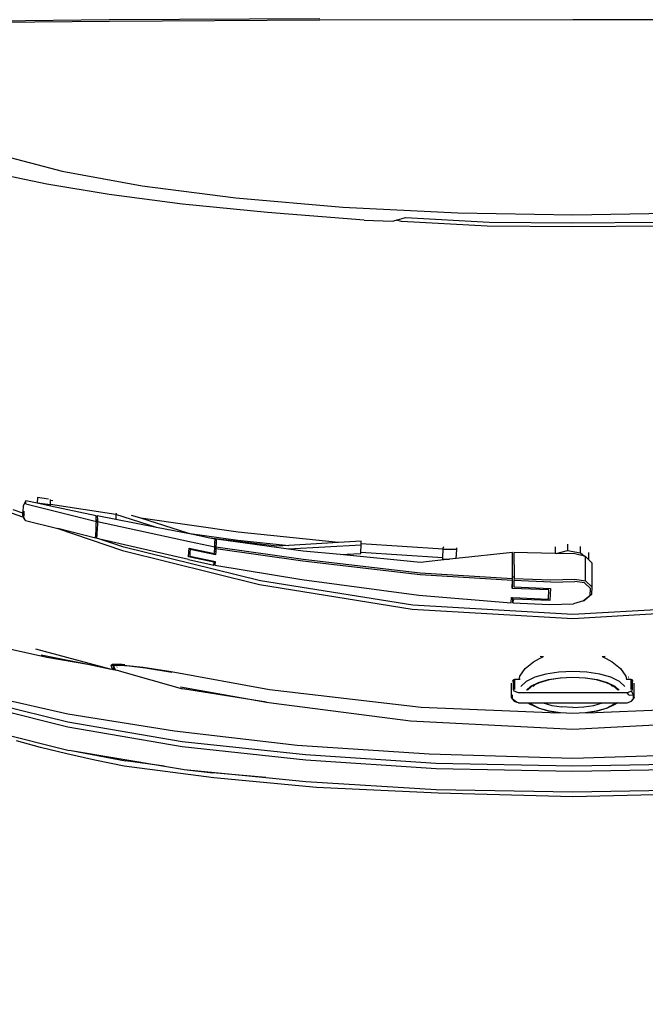
# Model space of a CAD drawing. Units: inches. Extents: x 22042254 to 25404563, y 17568978 to 17626777.
# Tile 22 of 45: x 22179830 to 22179852, y 17626194 to 17626227. Entities that reach past the tile are written whole.
import ezdxf

# ---------------------------------------------------------------- set-up
doc = ezdxf.new("R2010")
doc.units = ezdxf.units.IN
doc.header["$MEASUREMENT"] = 0
doc.layers.add('A-ANNO-DIMS', color=2, linetype='Continuous', lineweight=18)
doc.layers.add('A-SITE-VEHI', color=8, linetype='Continuous', lineweight=18)
doc.layers.add('Edges', color=250, linetype='Continuous')
doc.styles.get("Standard").update_dxf_attribs({"font": 'arial.ttf'})
doc.dimstyles.get("Standard").update_dxf_attribs({"dimtxt": 8, "dimasz": 0.18, "dimexe": 0.18, "dimexo": 0.0625, "dimgap": 0.09, "dimtad": 0, "dimtih": 1, "dimtoh": 1, "dimzin": 0, "dimdsep": 46, "dimlunit": 3, "dimtxsty": 'Standard', "dimcen": 0.09, "dimadec": 0, "dimazin": 0, "dimtfac": 1, "dimtofl": 0, "dimtmove": 0, "dimatfit": 3, "dimfxl": 1, "dimtolj": 1, "dimtzin": 0, "dimarcsym": 0})

# ---------------------------------------------------------------- blocks, each defined once
blk = doc.blocks.new('Nissan Qashqai pl')
at = {"layer": 'Edges'}
for p, q in [((11.05972, 12.11965), (11.05938, 11.92208)), ((11.5166, 12.04708), (11.52386, 11.92208)), ((11.52698, 11.92208), (11.51964, 12.0475)), ((11.61327, 11.92208), (11.60675, 12.04892)), ((11.60051, 11.93346), (11.59629, 12.04057)), ((11.63292, 12.0344), (11.63628, 11.92208)), ((11.64211, 11.92208), (11.63993, 12.02899)), ((11.64437, 12.02886), (11.64655, 11.92208)), ((11.66226, 11.92208), (11.66041, 12.02874)), ((11.66349, 12.02738), (11.66628, 11.92208)), ((11.21164, 11.92208), (11.21014, 12.01197)), ((11.22044, 11.98904), (11.22108, 11.92208)), ((11.21801, 11.92208), (11.21745, 11.98742)), ((11.57261, 11.96533), (11.57261, 11.96561)), ((11.57306, 11.96528), (11.57306, 11.96569)), ((11.57479, 11.96843), (11.57457, 11.96768)), ((11.58239, 11.96768), (11.57457, 11.96768)), ((11.57457, 11.96768), (11.57457, 11.96395)), ((11.57617, 11.96938), (11.57479, 11.96843)), ((11.57479, 11.96843), (11.58262, 11.96843)), ((11.58846, 11.97008), (11.57758, 11.97008)), ((11.58262, 11.96843), (11.58377, 11.96782)), ((11.58668, 11.96947), (11.58377, 11.96782)), ((11.58377, 11.96782), (11.58513, 11.96453)), ((11.58679, 11.96604), (11.58513, 11.96453)), ((11.58679, 11.96604), (11.58668, 11.96947)), ((11.58961, 11.96947), (11.58668, 11.96947)), ((11.58846, 11.97008), (11.58961, 11.96947)), ((11.5915, 11.96782), (11.58961, 11.96947)), ((11.5915, 11.96782), (11.59043, 11.96839)), ((11.59285, 11.96453), (11.5915, 11.96782)), ((11.56082, 11.95281), (11.56588, 11.95938)), ((11.56588, 11.95938), (11.57195, 11.96347)), ((11.57195, 11.96347), (11.57457, 11.96395)), ((11.57613, 11.95845), (11.57286, 11.95178)), ((11.57457, 11.96395), (11.57457, 11.96378)), ((11.57994, 11.96265), (11.57613, 11.95845)), ((11.57987, 11.95487), (11.58291, 11.95821)), ((11.58291, 11.95743), (11.58001, 11.95424)), ((11.58513, 11.96453), (11.58513, 11.87963)), ((11.59285, 11.95694), (11.59285, 11.96453)), ((11.55816, 11.94815), (11.56082, 11.95281)), ((11.57286, 11.95178), (11.57035, 11.94308)), ((11.57692, 11.94885), (11.57987, 11.95487)), ((11.57876, 11.95169), (11.57712, 11.94834)), ((11.58001, 11.95424), (11.57876, 11.95169)), ((11.57876, 11.95169), (11.57995, 11.953)), ((11.59285, 11.95694), (11.59412, 11.95487)), ((11.59285, 11.95657), (11.59285, 11.95694)), ((11.59319, 11.9559), (11.59285, 11.95657)), ((11.59285, 11.95626), (11.59285, 11.95657)), ((11.59285, 11.95626), (11.59319, 11.9559)), ((11.59285, 11.95549), (11.59285, 11.95626)), ((11.59398, 11.95424), (11.59285, 11.95549)), ((11.59285, 11.94526), (11.59285, 11.95549)), ((11.59319, 11.9559), (11.59412, 11.95487)), ((11.59688, 11.94834), (11.59398, 11.95424)), ((11.59412, 11.95487), (11.59707, 11.94885)), ((11.55654, 11.94509), (11.55639, 11.94749)), ((11.55654, 11.94509), (11.55816, 11.94815)), ((11.57035, 11.94308), (11.56877, 11.93295)), ((11.57466, 11.94101), (11.57692, 11.94885)), ((11.57712, 11.94834), (11.5749, 11.94065)), ((11.59285, 11.8989), (11.59285, 11.94526)), ((11.59478, 11.93858), (11.59285, 11.94526)), ((11.5991, 11.94065), (11.59688, 11.94834)), ((11.59707, 11.94885), (11.59933, 11.94101)), ((11.48106, 11.93457), (11.47554, 11.93456)), ((11.48106, 11.93457), (11.4786, 11.93206)), ((11.48349, 11.93703), (11.48106, 11.93457)), ((11.48349, 11.93703), (11.50222, 11.93704)), ((11.49744, 11.93207), (11.50222, 11.93704)), ((11.50349, 11.93588), (11.49907, 11.93132)), ((11.50222, 11.93704), (11.50812, 11.93671)), ((11.50889, 11.93558), (11.50349, 11.93588)), ((11.50812, 11.93671), (11.51287, 11.9312)), ((11.50889, 11.93558), (11.51321, 11.93053)), ((11.57324, 11.93188), (11.57466, 11.94101)), ((11.5749, 11.94065), (11.5735, 11.93169)), ((11.59602, 11.93062), (11.59478, 11.93858)), ((11.60049, 11.93169), (11.5991, 11.94065)), ((11.59933, 11.94101), (11.60051, 11.93346)), ((11.47578, 11.92803), (11.47062, 11.92803)), ((11.47398, 11.91798), (11.47578, 11.92803)), ((11.47578, 11.92803), (11.4784, 11.93124)), ((11.4784, 11.93124), (11.47657, 11.92368)), ((11.4786, 11.93206), (11.4784, 11.93124)), ((11.49744, 11.93207), (11.4786, 11.93206)), ((11.49621, 11.92369), (11.49744, 11.93207)), ((11.49907, 11.93132), (11.49795, 11.92364)), ((11.51321, 11.93053), (11.51287, 11.9312)), ((11.51321, 11.93053), (11.51543, 11.92267)), ((11.56877, 11.93295), (11.56823, 11.92208)), ((11.57275, 11.92208), (11.57324, 11.93188)), ((11.5735, 11.93169), (11.57302, 11.92208)), ((11.59645, 11.92208), (11.59602, 11.93062)), ((11.60097, 11.92208), (11.60049, 11.93169)), ((11.60051, 11.93346), (11.60076, 11.93188)), ((11.60076, 11.93188), (11.60124, 11.92208)), ((11.05938, 11.92208), (11.05972, 11.72451)), ((11.21014, 11.8322), (11.21164, 11.92208)), ((11.21745, 11.85674), (11.21801, 11.92208)), ((11.22108, 11.92208), (11.22044, 11.85512)), ((11.47657, 11.92368), (11.47622, 11.90912)), ((11.49689, 11.90495), (11.49621, 11.92369)), ((11.49859, 11.9049), (11.49795, 11.92364)), ((11.51606, 11.90392), (11.51543, 11.92267)), ((11.52386, 11.92208), (11.5166, 11.79708)), ((11.51964, 11.79666), (11.52698, 11.92208)), ((11.56823, 11.92208), (11.56877, 11.91121)), ((11.57324, 11.91228), (11.57275, 11.92208)), ((11.57302, 11.92208), (11.5735, 11.91247)), ((11.59645, 11.92208), (11.59602, 11.91354)), ((11.60049, 11.91247), (11.60097, 11.92208)), ((11.60124, 11.92208), (11.60076, 11.91228)), ((11.60675, 11.79524), (11.61327, 11.92208)), ((11.63628, 11.92208), (11.63292, 11.80976)), ((11.63993, 11.81518), (11.64211, 11.92208)), ((11.64655, 11.92208), (11.64437, 11.8153)), ((11.66041, 11.81542), (11.66226, 11.92208)), ((11.66628, 11.92208), (11.66349, 11.81678)), ((11.46896, 11.91798), (11.47398, 11.91798)), ((11.47622, 11.90912), (11.47398, 11.91798)), ((11.57466, 11.90315), (11.57324, 11.91228)), ((11.5735, 11.91247), (11.5749, 11.90351)), ((11.59478, 11.90558), (11.59602, 11.91354)), ((11.5991, 11.90351), (11.60049, 11.91247)), ((11.60076, 11.91228), (11.60051, 11.91071)), ((11.47102, 11.90825), (11.4762, 11.90826)), ((11.4762, 11.90826), (11.47542, 11.87608)), ((11.47622, 11.90912), (11.4762, 11.90826)), ((11.49565, 11.87616), (11.49689, 11.90495)), ((11.49859, 11.9049), (11.49735, 11.87612)), ((11.50223, 11.8759), (11.50346, 11.90468)), ((11.50346, 11.90468), (11.51299, 11.90415)), ((11.51299, 11.90415), (11.51176, 11.87537)), ((11.51483, 11.87514), (11.51606, 11.90392)), ((11.56877, 11.91121), (11.57035, 11.90108)), ((11.59285, 11.8989), (11.59478, 11.90558)), ((11.59629, 11.80359), (11.60051, 11.91071)), ((11.60051, 11.91071), (11.59933, 11.90315)), ((11.50462, 11.90341), (11.50341, 11.87505)), ((11.51177, 11.90301), (11.50462, 11.90341)), ((11.51058, 11.87508), (11.51177, 11.90301)), ((11.55639, 11.89667), (11.55654, 11.89907)), ((11.55816, 11.89601), (11.55654, 11.89907)), ((11.56082, 11.89135), (11.55816, 11.89601)), ((11.57035, 11.90108), (11.57286, 11.89238)), ((11.57692, 11.89531), (11.57466, 11.90315)), ((11.5749, 11.90351), (11.57712, 11.89582)), ((11.59285, 11.88868), (11.59285, 11.8989)), ((11.59688, 11.89582), (11.5991, 11.90351)), ((11.59933, 11.90315), (11.59707, 11.89531)), ((11.56588, 11.88478), (11.56082, 11.89135)), ((11.57286, 11.89238), (11.57613, 11.88571)), ((11.57987, 11.88929), (11.57692, 11.89531)), ((11.57712, 11.89582), (11.57876, 11.89248)), ((11.57995, 11.89116), (11.57876, 11.89248)), ((11.57876, 11.89248), (11.58001, 11.88992)), ((11.58291, 11.88595), (11.57987, 11.88929)), ((11.58001, 11.88992), (11.58291, 11.88673)), ((11.59285, 11.88868), (11.59398, 11.88992)), ((11.59285, 11.88722), (11.59412, 11.88929)), ((11.59285, 11.8879), (11.59285, 11.88868)), ((11.59285, 11.88759), (11.59319, 11.88827)), ((11.59319, 11.88827), (11.59285, 11.8879)), ((11.59412, 11.88929), (11.59319, 11.88827)), ((11.59398, 11.88992), (11.59688, 11.89582)), ((11.59707, 11.89531), (11.59412, 11.88929)), ((11.57195, 11.88069), (11.56588, 11.88478)), ((11.57261, 11.88057), (11.57195, 11.88069)), ((11.57261, 11.88057), (11.57261, 11.88076)), ((11.57306, 11.88049), (11.57261, 11.88057)), ((11.57306, 11.88049), (11.57306, 11.88081)), ((11.57457, 11.88096), (11.57457, 11.88021)), ((11.57613, 11.88571), (11.57994, 11.88151)), ((11.59285, 11.88759), (11.59285, 11.8879)), ((11.59285, 11.88722), (11.59285, 11.88759)), ((11.59285, 11.87963), (11.59285, 11.88722)), ((11.49563, 11.87496), (11.47539, 11.87488)), ((11.47539, 11.87488), (11.4801, 11.83099)), ((11.47542, 11.87608), (11.49451, 11.87616)), ((11.49133, 11.80278), (11.49563, 11.87496)), ((11.49732, 11.87492), (11.49295, 11.80271)), ((11.49449, 11.87502), (11.49451, 11.87616)), ((11.50341, 11.87505), (11.49449, 11.87502)), ((11.49451, 11.87616), (11.49565, 11.87616)), ((11.49732, 11.87492), (11.49563, 11.87496)), ((11.49565, 11.87616), (11.49735, 11.87612)), ((11.50339, 11.87463), (11.49732, 11.87492)), ((11.49735, 11.87612), (11.50223, 11.8759)), ((11.50341, 11.87505), (11.50339, 11.87463)), ((11.50884, 11.80182), (11.5148, 11.87394)), ((11.51054, 11.87423), (11.51058, 11.87508)), ((11.5148, 11.87394), (11.51054, 11.87423)), ((11.51472, 11.8751), (11.51058, 11.87508)), ((11.51176, 11.87537), (11.51472, 11.87515)), ((11.51472, 11.87515), (11.51472, 11.8751)), ((11.51472, 11.87515), (11.51483, 11.87514)), ((11.51483, 11.87514), (11.51472, 11.8751)), ((11.57457, 11.88021), (11.57306, 11.88049)), ((11.57457, 11.88021), (11.57457, 11.87648)), ((11.57457, 11.87648), (11.58239, 11.87648)), ((11.57457, 11.87648), (11.57479, 11.87573)), ((11.58262, 11.87573), (11.57479, 11.87573)), ((11.57479, 11.87573), (11.57617, 11.87478)), ((11.58846, 11.87408), (11.57758, 11.87408)), ((11.58377, 11.87635), (11.58262, 11.87573)), ((11.58513, 11.87963), (11.58377, 11.87635)), ((11.58668, 11.87469), (11.58961, 11.87469)), ((11.58961, 11.87469), (11.58846, 11.87408)), ((11.58961, 11.87469), (11.5915, 11.87635)), ((11.59043, 11.87577), (11.58961, 11.87469)), ((11.59221, 11.87812), (11.59043, 11.87577)), ((11.59043, 11.87577), (11.5915, 11.87635)), ((11.5915, 11.87635), (11.59221, 11.87812)), ((11.59285, 11.87963), (11.59221, 11.87812)), ((11.2139, 11.7914), (11.21745, 11.85674)), ((11.22044, 11.85512), (11.21682, 11.78816)), ((11.20565, 11.74231), (11.21014, 11.8322)), ((11.47305, 11.83139), (11.47165, 11.83144)), ((11.47305, 11.83139), (11.473, 11.82087)), ((11.4801, 11.83099), (11.47305, 11.83139)), ((11.4801, 11.83099), (11.48065, 11.82584)), ((11.47281, 11.82086), (11.46872, 11.75675)), ((11.47111, 11.82093), (11.47189, 11.82089)), ((11.47281, 11.82086), (11.47189, 11.82089)), ((11.473, 11.82087), (11.47281, 11.82086)), ((11.47916, 11.8205), (11.473, 11.82087)), ((11.47508, 11.75641), (11.47919, 11.82046)), ((11.47919, 11.82046), (11.47916, 11.8205)), ((11.48062, 11.82044), (11.47919, 11.82046)), ((11.48062, 11.82044), (11.48065, 11.82584)), ((11.48065, 11.82584), (11.4831, 11.803)), ((11.63327, 11.71316), (11.63993, 11.81518)), ((11.64437, 11.8153), (11.63768, 11.7134)), ((11.65425, 11.71357), (11.66041, 11.81542)), ((11.66349, 11.81678), (11.65888, 11.72193)), ((11.63292, 11.80976), (11.62604, 11.70665)), ((11.4831, 11.803), (11.47707, 11.74042)), ((11.4805, 11.71128), (11.49133, 11.80278)), ((11.49295, 11.80271), (11.48212, 11.71121)), ((11.49642, 11.71041), (11.50884, 11.80182)), ((11.5166, 11.79708), (11.49761, 11.67796)), ((11.50045, 11.6772), (11.51964, 11.79666)), ((11.58235, 11.68521), (11.59629, 11.80359)), ((11.21579, 11.78424), (11.2139, 11.7914)), ((11.5932, 11.68852), (11.60675, 11.79524)), ((11.21682, 11.78816), (11.21579, 11.78424)), ((11.21585, 11.78401), (11.21579, 11.78424)), ((11.21682, 11.78816), (11.21585, 11.78401)), ((11.21658, 11.78121), (11.21585, 11.78401)), ((11.21586, 11.75915), (11.21658, 11.78121)), ((11.21586, 11.75915), (11.20997, 11.68347)), ((11.46872, 11.75675), (11.46649, 11.75682)), ((11.46649, 11.75682), (11.46757, 11.73891)), ((11.46975, 11.75671), (11.46872, 11.75675)), ((11.46975, 11.75671), (11.47273, 11.69994)), ((11.47508, 11.75641), (11.46975, 11.75671)), ((11.47611, 11.75636), (11.47508, 11.75641)), ((11.47707, 11.74042), (11.47611, 11.75636)), ((11.19842, 11.65867), (11.20565, 11.74231)), ((11.46757, 11.73891), (11.45941, 11.6607)), ((11.46757, 11.73891), (11.46992, 11.70014)), ((11.47707, 11.74042), (11.47428, 11.71144)), ((11.0586, 11.72441), (11.05947, 11.55994)), ((11.05972, 11.72451), (11.06059, 11.56009)), ((11.65888, 11.72193), (11.65143, 11.64152)), ((11.47428, 11.71144), (11.47273, 11.69994)), ((11.6229, 11.61679), (11.63327, 11.71316)), ((11.63768, 11.7134), (11.62719, 11.61693)), ((11.65114, 11.68233), (11.65425, 11.71357)), ((11.47094, 11.64327), (11.4805, 11.71128)), ((11.48212, 11.71121), (11.47257, 11.6432)), ((11.48539, 11.64249), (11.49642, 11.71041)), ((11.62604, 11.70665), (11.61495, 11.61084)), ((11.47273, 11.69994), (11.46512, 11.64343)), ((11.46576, 11.66035), (11.46992, 11.70014)), ((11.46992, 11.70014), (11.47047, 11.69095)), ((11.47047, 11.69095), (11.46419, 11.63849)), ((11.59218, 11.68277), (11.5932, 11.68852)), ((11.20997, 11.68347), (11.2033, 11.61723)), ((11.56846, 11.60829), (11.58235, 11.68521)), ((11.58021, 11.61555), (11.59218, 11.68277)), ((11.59218, 11.68277), (11.58179, 11.61717)), ((11.64478, 11.61839), (11.65114, 11.68233)), ((11.65114, 11.68233), (11.64749, 11.64092)), ((11.49761, 11.67796), (11.47115, 11.57128)), ((11.47375, 11.5702), (11.50045, 11.6772)), ((11.18907, 11.58559), (11.19842, 11.65867)), ((11.45941, 11.6607), (11.44866, 11.58459)), ((11.46024, 11.62121), (11.46576, 11.66035)), ((11.46505, 11.64255), (11.46419, 11.63849)), ((11.46792, 11.64248), (11.46505, 11.64255)), ((11.46512, 11.64343), (11.46801, 11.64335)), ((11.46687, 11.62247), (11.47088, 11.64239)), ((11.46801, 11.64335), (11.46792, 11.64248)), ((11.47088, 11.64239), (11.46792, 11.64248)), ((11.46801, 11.64335), (11.47094, 11.64327)), ((11.47252, 11.64233), (11.47088, 11.64239)), ((11.47094, 11.64327), (11.47257, 11.6432)), ((11.47212, 11.62223), (11.47625, 11.64214)), ((11.47439, 11.64223), (11.47252, 11.64233)), ((11.47257, 11.6432), (11.47449, 11.6431)), ((11.47727, 11.64296), (11.47315, 11.62305)), ((11.47439, 11.64223), (11.47449, 11.6431)), ((11.47625, 11.64214), (11.47439, 11.64223)), ((11.47449, 11.6431), (11.47727, 11.64296)), ((11.48226, 11.64167), (11.48244, 11.64254)), ((11.48244, 11.64254), (11.48247, 11.64267)), ((11.48535, 11.64246), (11.48244, 11.64254)), ((11.48247, 11.64267), (11.48535, 11.64246)), ((11.48539, 11.64249), (11.48535, 11.64246)), ((11.46419, 11.63849), (11.46114, 11.62406)), ((11.47827, 11.62277), (11.48226, 11.64167)), ((11.48298, 11.64165), (11.47879, 11.62186)), ((11.48098, 11.62171), (11.48532, 11.64161)), ((11.48226, 11.64167), (11.48298, 11.64165)), ((11.483, 11.64176), (11.48298, 11.64165)), ((11.48532, 11.64161), (11.483, 11.64176)), ((11.65143, 11.64152), (11.64217, 11.57162)), ((11.64478, 11.61839), (11.64749, 11.64092)), ((11.46024, 11.62121), (11.44866, 11.58459)), ((11.45125, 11.55073), (11.46687, 11.62247)), ((11.46083, 11.62261), (11.45585, 11.5969)), ((11.46114, 11.62406), (11.46024, 11.62121)), ((11.46114, 11.62406), (11.46083, 11.62261)), ((11.48098, 11.62171), (11.4649, 11.55261)), ((11.47495, 11.62207), (11.47212, 11.62223)), ((11.47315, 11.62305), (11.47515, 11.62294)), ((11.47495, 11.62207), (11.47515, 11.62294)), ((11.47879, 11.62186), (11.47495, 11.62207)), ((11.47515, 11.62294), (11.47827, 11.62277)), ((11.2033, 11.61723), (11.19582, 11.55976)), ((11.56776, 11.56755), (11.58179, 11.61717)), ((11.60765, 11.5276), (11.6229, 11.61679)), ((11.62719, 11.61693), (11.61178, 11.52762)), ((11.64227, 11.603), (11.64462, 11.61709)), ((11.64462, 11.61709), (11.64478, 11.61839)), ((11.56499, 11.58644), (11.56846, 11.60829)), ((11.56905, 11.60888), (11.56563, 11.58822)), ((11.61495, 11.61084), (11.6016, 11.52761)), ((11.45585, 11.5969), (11.44582, 11.56516)), ((11.45585, 11.5969), (11.44965, 11.56495)), ((11.63012, 11.53004), (11.64227, 11.603)), ((11.64227, 11.603), (11.63807, 11.5726)), ((11.17758, 11.52307), (11.18907, 11.58559)), ((11.44866, 11.58459), (11.44723, 11.58007)), ((11.56356, 11.57357), (11.56499, 11.58644)), ((11.56563, 11.58822), (11.56415, 11.57536)), ((11.44723, 11.58007), (11.44639, 11.57739)), ((11.56335, 11.56843), (11.56356, 11.57357)), ((11.56415, 11.57536), (11.56375, 11.56794)), ((11.45676, 11.51971), (11.47375, 11.5702)), ((11.47115, 11.57128), (11.4649, 11.55261)), ((11.56255, 11.56701), (11.56268, 11.56956)), ((11.56271, 11.56245), (11.56255, 11.56701)), ((11.56268, 11.56956), (11.56259, 11.5697)), ((11.56268, 11.56956), (11.5628, 11.57206)), ((11.56335, 11.56843), (11.56268, 11.56956)), ((11.56325, 11.56586), (11.56335, 11.56843)), ((11.56334, 11.56271), (11.56325, 11.56586)), ((11.56368, 11.56788), (11.56335, 11.56843)), ((11.56375, 11.56794), (11.56392, 11.56325)), ((11.56487, 11.5659), (11.56469, 11.5662)), ((11.56704, 11.56455), (11.56739, 11.56625)), ((11.56712, 11.56458), (11.56763, 11.56708)), ((11.56717, 11.5646), (11.56763, 11.56708)), ((11.56745, 11.56646), (11.56739, 11.56625)), ((11.56763, 11.56708), (11.56776, 11.56755)), ((11.63012, 11.53004), (11.63807, 11.5726)), ((11.64217, 11.57162), (11.63751, 11.54857)), ((11.05947, 11.55994), (11.06074, 11.45082)), ((11.06059, 11.56009), (11.06182, 11.4509)), ((11.19582, 11.55976), (11.18773, 11.51111)), ((11.44575, 11.56516), (11.43801, 11.51398)), ((11.4448, 11.5652), (11.44575, 11.56516)), ((11.44575, 11.56516), (11.44582, 11.56516)), ((11.44582, 11.56516), (11.44965, 11.56495)), ((11.44965, 11.56495), (11.44685, 11.5505)), ((11.55053, 11.5023), (11.56648, 11.56144)), ((11.56334, 11.56271), (11.56271, 11.56245)), ((11.56338, 11.56129), (11.56271, 11.56245)), ((11.56273, 11.5431), (11.56648, 11.56144)), ((11.56609, 11.56386), (11.56334, 11.56271)), ((11.56338, 11.56129), (11.56334, 11.56271)), ((11.56583, 11.56223), (11.56338, 11.56129)), ((11.56392, 11.56325), (11.56429, 11.56338)), ((11.56429, 11.56338), (11.56596, 11.56408)), ((11.56609, 11.56386), (11.56583, 11.56223)), ((11.56616, 11.56236), (11.56583, 11.56223)), ((11.56596, 11.56408), (11.56616, 11.56417)), ((11.56609, 11.56386), (11.56596, 11.56408)), ((11.56613, 11.56388), (11.56609, 11.56386)), ((11.56618, 11.56418), (11.56613, 11.56388)), ((11.56613, 11.56388), (11.56616, 11.56417)), ((11.56613, 11.56388), (11.56645, 11.5641)), ((11.56665, 11.56424), (11.56616, 11.56236)), ((11.56616, 11.56417), (11.56618, 11.56418)), ((11.56616, 11.56236), (11.56645, 11.5641)), ((11.56661, 11.56253), (11.56616, 11.56236)), ((11.56618, 11.56418), (11.56648, 11.56431)), ((11.56645, 11.5641), (11.56648, 11.56431)), ((11.56645, 11.5641), (11.56665, 11.56424)), ((11.56648, 11.56431), (11.56669, 11.5644)), ((11.56679, 11.56261), (11.56648, 11.56144)), ((11.56661, 11.56253), (11.56704, 11.56455)), ((11.56671, 11.56257), (11.56661, 11.56253)), ((11.56665, 11.56424), (11.56688, 11.56448)), ((11.56669, 11.5644), (11.56665, 11.56424)), ((11.56669, 11.5644), (11.56688, 11.56448)), ((11.56671, 11.56257), (11.56712, 11.56458)), ((11.56679, 11.56261), (11.56671, 11.56257)), ((11.56717, 11.5646), (11.56679, 11.56261)), ((11.56688, 11.56448), (11.56704, 11.56455)), ((11.56704, 11.56455), (11.56712, 11.56458)), ((11.56712, 11.56458), (11.56717, 11.5646)), ((11.44685, 11.5505), (11.44997, 11.55066)), ((11.44983, 11.54978), (11.44997, 11.55066)), ((11.44997, 11.55066), (11.45125, 11.55073)), ((11.45125, 11.55073), (11.4529, 11.55066)), ((11.4529, 11.55066), (11.45711, 11.55045)), ((11.45711, 11.55045), (11.45994, 11.5503)), ((11.45983, 11.54978), (11.45994, 11.5503)), ((11.46402, 11.54999), (11.45983, 11.54978)), ((11.45994, 11.5503), (11.46197, 11.55018)), ((11.46197, 11.55018), (11.46404, 11.55004)), ((11.46402, 11.54999), (11.46375, 11.54918)), ((11.46404, 11.55004), (11.46402, 11.54999)), ((11.46423, 11.55), (11.46402, 11.54999)), ((11.46404, 11.55004), (11.46423, 11.55)), ((11.46423, 11.55), (11.46424, 11.55003)), ((11.4643, 11.55002), (11.46423, 11.55)), ((11.4649, 11.55261), (11.4643, 11.55002)), ((11.43747, 11.49463), (11.45125, 11.54985)), ((11.44684, 11.54963), (11.43914, 11.51392)), ((11.44983, 11.54978), (11.44684, 11.54963)), ((11.45125, 11.54985), (11.44983, 11.54978)), ((11.4529, 11.54978), (11.45125, 11.54985)), ((11.45711, 11.54958), (11.4529, 11.54978)), ((11.46429, 11.54915), (11.45676, 11.51971)), ((11.46197, 11.5493), (11.45711, 11.54958)), ((11.46375, 11.54918), (11.46197, 11.5493)), ((11.46429, 11.54915), (11.46375, 11.54918)), ((11.55533, 11.50682), (11.56273, 11.5431)), ((11.55707, 11.51104), (11.56273, 11.5431)), ((11.63751, 11.54857), (11.63276, 11.52672)), ((11.6016, 11.52761), (11.58664, 11.46068)), ((11.58843, 11.44985), (11.60765, 11.5276)), ((11.61178, 11.52762), (11.59225, 11.44945)), ((11.61272, 11.45895), (11.62966, 11.52759)), ((11.62966, 11.52759), (11.63012, 11.53004)), ((11.16395, 11.47112), (11.17758, 11.52307)), ((11.45032, 11.49453), (11.45676, 11.51971)), ((11.63276, 11.52672), (11.62771, 11.50627)), ((11.43371, 11.51238), (11.43251, 11.50378)), ((11.43475, 11.51409), (11.43403, 11.51411)), ((11.43501, 11.51584), (11.43475, 11.51409)), ((11.43801, 11.51398), (11.43475, 11.51409)), ((11.4382, 11.51397), (11.43676, 11.50364)), ((11.43914, 11.51392), (11.43692, 11.50363)), ((11.4382, 11.51397), (11.43801, 11.51398)), ((11.43914, 11.51392), (11.4382, 11.51397)), ((11.18773, 11.51111), (11.17906, 11.46956)), ((11.43251, 11.50378), (11.43676, 11.50364)), ((11.43251, 11.50378), (11.4369, 11.50353)), ((11.54814, 11.47101), (11.55707, 11.51104)), ((11.62771, 11.50627), (11.62241, 11.48743)), ((11.4369, 11.50353), (11.435, 11.49469)), ((11.43676, 11.50364), (11.43692, 11.50363)), ((11.43692, 11.50363), (11.4369, 11.50353)), ((11.435, 11.49469), (11.43896, 11.49272)), ((11.43747, 11.49463), (11.435, 11.49469)), ((11.43896, 11.49272), (11.44373, 11.49245)), ((11.44474, 11.49242), (11.44218, 11.48476)), ((11.44507, 11.49341), (11.44316, 11.49351)), ((11.44373, 11.49245), (11.44491, 11.49291)), ((11.44474, 11.49242), (11.44373, 11.49245)), ((11.44453, 11.48334), (11.44778, 11.49299)), ((11.44491, 11.49291), (11.44474, 11.49242)), ((11.4462, 11.49239), (11.44474, 11.49242)), ((11.44507, 11.49341), (11.44491, 11.49291)), ((11.44491, 11.49291), (11.44606, 11.49335)), ((11.44606, 11.49335), (11.44507, 11.49341)), ((11.44786, 11.49325), (11.44606, 11.49335)), ((11.44786, 11.49325), (11.4462, 11.49239)), ((11.44778, 11.49299), (11.4462, 11.49239)), ((11.45018, 11.49392), (11.44778, 11.49299)), ((11.44794, 11.49325), (11.44786, 11.49325)), ((11.45032, 11.49453), (11.44794, 11.49325)), ((11.45018, 11.49392), (11.45032, 11.49453))]:
    blk.add_line(p, q, dxfattribs=at)
blk = doc.blocks.new('CAR')
blk.add_blockref('Nissan Qashqai pl', (-9.74328, -11.91512))
blk = doc.blocks.new('*D59')
at = {"layer": 'A-ANNO-DIMS', "color": 0, "lineweight": -2, "transparency": 16777216}
for p, q in [((22179802.402, 17626200.497), (22179802.402, 17626171.756)), ((22179895.926, 17626200.497), (22179895.926, 17626171.756)), ((22179802.582, 17626171.936), (22179829.153, 17626171.936)), ((22179895.746, 17626171.936), (22179869.175, 17626171.936))]:
    blk.add_line(p, q, dxfattribs=at)
at = {"layer": 'A-ANNO-DIMS', "color": 0, "transparency": 16777216}
for points in [[(22179802.582, 17626171.966), (22179802.582, 17626171.906), (22179802.402, 17626171.936)], [(22179895.746, 17626171.966), (22179895.746, 17626171.906), (22179895.926, 17626171.936)]]:
    blk.add_solid(points, dxfattribs=at)
at = {"layer": 'Defpoints', "color": 0, "transparency": 16777216}
for p in [(22179802.402, 17626200.559), (22179895.926, 17626200.559), (22179895.926, 17626171.936)]:
    blk.add_point(p, dxfattribs=at)
at = {"layer": 'A-ANNO-DIMS', "color": 0, "transparency": 16777216, "insert": (22179849.164, 17626171.936), "char_height": 8, "attachment_point": 5}
blk.add_mtext('\\A1;7\'-9 1/2"', dxfattribs=at)

msp = doc.modelspace()

# ---------------------------------------------------------------- block references
at = {"layer": 'A-SITE-VEHI', "xscale": 43.56002006885659, "yscale": 43.56002006885659, "zscale": 43.56002006885659, "rotation": 270}
msp.add_blockref('CAR', (22179848.861, 17626284.325), dxfattribs=at)

# ---------------------------------------------------------------- dimensions: what is measured, and where the dimension line sits
at = {"layer": 'A-ANNO-DIMS'}
dim = msp.add_linear_dim(base=(22179895.926, 17626171.936), p1=(22179802.402, 17626200.559), p2=(22179895.926, 17626200.559), dimstyle='Standard', override={"dimdec": 1, "dimlfac": 1, "dimrnd": 0, "dimzin": 1, "dimdsep": 46, "dimlunit": 4, "dimfrac": 2}, dxfattribs=at)
dim.commit()
dim.dimension.update_dxf_attribs({"geometry": '*D59', "text_midpoint": (22179849.164, 17626171.936)})

doc.saveas('drawing.dxf')
